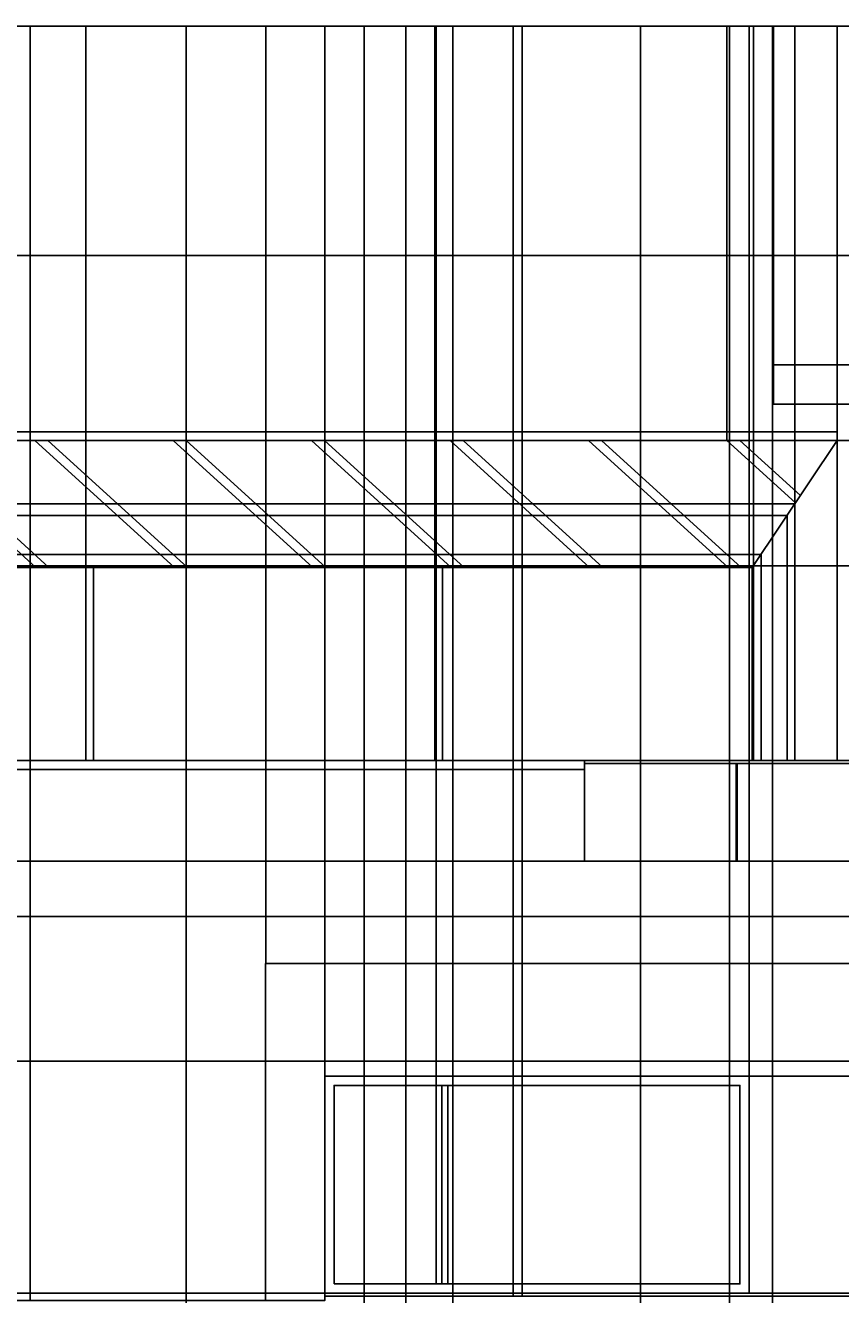
# Model space of a CAD drawing. Units: feet. Extents: x 2193 to 3502, y 890 to 1601.
# Tile 16 of 17: x 3069 to 3283, y 1268 to 1601. Entities that reach past the tile are written whole.
import ezdxf

# ---------------------------------------------------------------- set-up
doc = ezdxf.new("R2010")
doc.units = ezdxf.units.FT
doc.layers.add('A-ANNO-DIMS', color=2, linetype='Continuous', lineweight=18)
doc.layers.add('A-ELEV', color=7, linetype='Continuous', lineweight=25)
doc.styles.get("Standard").update_dxf_attribs({"font": 'arial.ttf'})
doc.dimstyles.get("Standard").update_dxf_attribs({"dimtxt": 0.18, "dimasz": 0.18, "dimexe": 0.18, "dimexo": 0.0625, "dimgap": 0.09, "dimtad": 0, "dimtih": 1, "dimtoh": 1, "dimdec": 0, "dimzin": 0, "dimdsep": 46, "dimlunit": 3, "dimtxsty": 'Standard', "dimcen": 0.09, "dimadec": 0, "dimazin": 0, "dimtfac": 1, "dimtdec": 0, "dimtofl": 0, "dimtmove": 0, "dimatfit": 3, "dimfxl": 1, "dimtolj": 1, "dimtzin": 0, "dimarcsym": 0})

# ---------------------------------------------------------------- blocks, each defined once
blk = doc.blocks.new('*D13')
at = {"layer": 'A-ANNO-DIMS', "color": 0, "lineweight": -2, "transparency": 16777216}
for p, q in [((2934.37, 950.89), (2934.37, 1601.47)), ((2934.55, 1601.29), (3186.64, 1601.29)), ((3439.51, 1601.29), (3187.43, 1601.29)), ((3439.69, 1541.11), (3439.69, 1601.47))]:
    blk.add_line(p, q, dxfattribs=at)
at = {"layer": 'A-ANNO-DIMS', "color": 0, "transparency": 16777216}
for points in [[(2934.55, 1601.32), (2934.55, 1601.26), (2934.37, 1601.29)], [(3439.51, 1601.32), (3439.51, 1601.26), (3439.69, 1601.29)]]:
    blk.add_solid(points, dxfattribs=at)
at = {"layer": 'Defpoints', "color": 0, "transparency": 16777216}
for p in [(3439.69, 1601.29), (3439.69, 1541.04), (2934.37, 950.82)]:
    blk.add_point(p, dxfattribs=at)
at = {"layer": 'A-ANNO-DIMS', "color": 0, "transparency": 16777216, "insert": (3187.03, 1601.29), "char_height": 0.18, "attachment_point": 5}
blk.add_mtext('\\A1;505.3', dxfattribs=at)
blk = doc.blocks.new('*D31')
at = {"layer": 'A-ANNO-DIMS', "color": 0, "lineweight": -2, "transparency": 16777216}
for p, q in [((2760.54, 1541.04), (3501.85, 1541.04)), ((3501.67, 1540.86), (3501.67, 1246.12)), ((3501.67, 951), (3501.67, 1245.75)), ((2762.27, 950.82), (3501.85, 950.82))]:
    blk.add_line(p, q, dxfattribs=at)
at = {"layer": 'A-ANNO-DIMS', "color": 0, "transparency": 16777216}
for points in [[(3501.64, 1540.86), (3501.7, 1540.86), (3501.67, 1541.04)], [(3501.64, 951), (3501.7, 951), (3501.67, 950.82)]]:
    blk.add_solid(points, dxfattribs=at)
at = {"layer": 'Defpoints', "color": 0, "transparency": 16777216}
for p in [(2760.47, 1541.04), (3501.67, 1541.04), (2762.2, 950.82)]:
    blk.add_point(p, dxfattribs=at)
at = {"layer": 'A-ANNO-DIMS', "color": 0, "transparency": 16777216, "insert": (3501.67, 1245.93), "char_height": 0.18, "attachment_point": 5}
blk.add_mtext('\\A1;590.2', dxfattribs=at)
blk = doc.blocks.new('*D43')
at = {"layer": 'A-ANNO-DIMS', "color": 0, "lineweight": -2, "transparency": 16777216}
for p, q in [((3265.39, 1512.46), (3265.39, 1601.47)), ((3265.57, 1601.29), (3273.35, 1601.29)), ((3281.9, 1601.29), (3274.12, 1601.29)), ((3282.08, 1502.14), (3282.08, 1601.47))]:
    blk.add_line(p, q, dxfattribs=at)
at = {"layer": 'A-ANNO-DIMS', "color": 0, "transparency": 16777216}
for points in [[(3265.57, 1601.32), (3265.57, 1601.26), (3265.39, 1601.29)], [(3281.9, 1601.32), (3281.9, 1601.26), (3282.08, 1601.29)]]:
    blk.add_solid(points, dxfattribs=at)
at = {"layer": 'Defpoints', "color": 0, "transparency": 16777216}
for p in [(3282.08, 1601.29), (3265.39, 1512.4), (3282.08, 1502.08)]:
    blk.add_point(p, dxfattribs=at)
at = {"layer": 'A-ANNO-DIMS', "color": 0, "transparency": 16777216, "insert": (3273.74, 1601.29), "char_height": 0.18, "attachment_point": 5}
blk.add_mtext('\\A1;16.69', dxfattribs=at)
blk = doc.blocks.new('*D44')
at = {"layer": 'A-ANNO-DIMS', "color": 0, "lineweight": -2, "transparency": 16777216}
for p, q in [((3282.08, 1502.14), (3282.08, 1601.47)), ((3282.26, 1601.29), (3330.07, 1601.29)), ((3378.67, 1601.29), (3330.86, 1601.29)), ((3378.85, 1502.14), (3378.85, 1601.47))]:
    blk.add_line(p, q, dxfattribs=at)
at = {"layer": 'A-ANNO-DIMS', "color": 0, "transparency": 16777216}
for points in [[(3282.26, 1601.32), (3282.26, 1601.26), (3282.08, 1601.29)], [(3378.67, 1601.32), (3378.67, 1601.26), (3378.85, 1601.29)]]:
    blk.add_solid(points, dxfattribs=at)
at = {"layer": 'Defpoints', "color": 0, "transparency": 16777216}
for p in [(3378.85, 1601.29), (3282.08, 1502.08), (3378.85, 1502.08)]:
    blk.add_point(p, dxfattribs=at)
at = {"layer": 'A-ANNO-DIMS', "color": 0, "transparency": 16777216, "insert": (3330.47, 1601.29), "char_height": 0.18, "attachment_point": 5}
blk.add_mtext('\\A1;96.77', dxfattribs=at)
blk = doc.blocks.new('*D48')
at = {"layer": 'A-ANNO-DIMS', "color": 0, "lineweight": -2, "transparency": 16777216}
for p, q in [((2965.72, 1494.87), (2965.72, 1601.47)), ((2965.9, 1601.29), (3123.44, 1601.29)), ((3281.9, 1601.29), (3124.36, 1601.29)), ((3282.08, 1494.87), (3282.08, 1601.47))]:
    blk.add_line(p, q, dxfattribs=at)
at = {"layer": 'A-ANNO-DIMS', "color": 0, "transparency": 16777216}
for points in [[(2965.9, 1601.32), (2965.9, 1601.26), (2965.72, 1601.29)], [(3281.9, 1601.32), (3281.9, 1601.26), (3282.08, 1601.29)]]:
    blk.add_solid(points, dxfattribs=at)
at = {"layer": 'Defpoints', "color": 0, "transparency": 16777216}
for p in [(3282.08, 1601.29), (2965.72, 1494.8), (3282.08, 1494.8)]:
    blk.add_point(p, dxfattribs=at)
at = {"layer": 'A-ANNO-DIMS', "color": 0, "transparency": 16777216, "insert": (3123.9, 1601.29), "char_height": 0.18, "attachment_point": 5}
blk.add_mtext('\\A1;316.36', dxfattribs=at)
blk = doc.blocks.new('*D50')
at = {"layer": 'A-ANNO-DIMS', "color": 0, "lineweight": -2, "transparency": 16777216}
for p, q in [((3260.1, 1459.67), (3260.1, 1601.47)), ((3260.28, 1601.29), (3270.7, 1601.29)), ((3281.9, 1601.29), (3271.49, 1601.29)), ((3282.08, 1492.58), (3282.08, 1601.47))]:
    blk.add_line(p, q, dxfattribs=at)
at = {"layer": 'A-ANNO-DIMS', "color": 0, "transparency": 16777216}
for points in [[(3260.28, 1601.32), (3260.28, 1601.26), (3260.1, 1601.29)], [(3281.9, 1601.32), (3281.9, 1601.26), (3282.08, 1601.29)]]:
    blk.add_solid(points, dxfattribs=at)
at = {"layer": 'Defpoints', "color": 0, "transparency": 16777216}
for p in [(3282.08, 1601.29), (3282.08, 1492.51), (3260.1, 1459.6)]:
    blk.add_point(p, dxfattribs=at)
at = {"layer": 'A-ANNO-DIMS', "color": 0, "transparency": 16777216, "insert": (3271.09, 1601.29), "char_height": 0.18, "attachment_point": 5}
blk.add_mtext('\\A1;21.98', dxfattribs=at)
blk = doc.blocks.new('*D51')
at = {"layer": 'A-ANNO-DIMS', "color": 0, "lineweight": -2, "transparency": 16777216}
for p, q in [((2965.78, 1492.51), (3501.85, 1492.51)), ((3501.67, 1492.33), (3501.67, 1476.24)), ((3501.67, 1459.78), (3501.67, 1475.88)), ((3001.96, 1459.6), (3501.85, 1459.6))]:
    blk.add_line(p, q, dxfattribs=at)
at = {"layer": 'A-ANNO-DIMS', "color": 0, "transparency": 16777216}
for points in [[(3501.64, 1492.33), (3501.7, 1492.33), (3501.67, 1492.51)], [(3501.64, 1459.78), (3501.7, 1459.78), (3501.67, 1459.6)]]:
    blk.add_solid(points, dxfattribs=at)
at = {"layer": 'Defpoints', "color": 0, "transparency": 16777216}
for p in [(2965.72, 1492.51), (3501.67, 1492.51), (3001.89, 1459.6)]:
    blk.add_point(p, dxfattribs=at)
at = {"layer": 'A-ANNO-DIMS', "color": 0, "transparency": 16777216, "insert": (3501.67, 1476.06), "char_height": 0.18, "attachment_point": 5}
blk.add_mtext('\\A1;32.91', dxfattribs=at)
blk = doc.blocks.new('*D54')
at = {"layer": 'A-ANNO-DIMS', "color": 0, "lineweight": -2, "transparency": 16777216}
for p, q in [((3002.38, 1408.54), (3002.38, 1601.47)), ((3002.56, 1601.29), (3043.2, 1601.29)), ((3084.62, 1601.29), (3043.99, 1601.29)), ((3084.8, 1408.54), (3084.8, 1601.47))]:
    blk.add_line(p, q, dxfattribs=at)
at = {"layer": 'A-ANNO-DIMS', "color": 0, "transparency": 16777216}
for points in [[(3002.56, 1601.32), (3002.56, 1601.26), (3002.38, 1601.29)], [(3084.62, 1601.32), (3084.62, 1601.26), (3084.8, 1601.29)]]:
    blk.add_solid(points, dxfattribs=at)
at = {"layer": 'Defpoints', "color": 0, "transparency": 16777216}
for p in [(3084.8, 1601.29), (3002.38, 1408.48), (3084.8, 1408.48)]:
    blk.add_point(p, dxfattribs=at)
at = {"layer": 'A-ANNO-DIMS', "color": 0, "transparency": 16777216, "insert": (3043.59, 1601.29), "char_height": 0.18, "attachment_point": 5}
blk.add_mtext('\\A1;82.42', dxfattribs=at)
blk = doc.blocks.new('*D55')
at = {"layer": 'A-ANNO-DIMS', "color": 0, "lineweight": -2, "transparency": 16777216}
for p, q in [((3084.8, 1408.54), (3084.8, 1601.47)), ((3084.98, 1601.29), (3130.23, 1601.29)), ((3176.26, 1601.29), (3131.01, 1601.29)), ((3176.44, 1408.54), (3176.44, 1601.47))]:
    blk.add_line(p, q, dxfattribs=at)
at = {"layer": 'A-ANNO-DIMS', "color": 0, "transparency": 16777216}
for points in [[(3084.98, 1601.32), (3084.98, 1601.26), (3084.8, 1601.29)], [(3176.26, 1601.32), (3176.26, 1601.26), (3176.44, 1601.29)]]:
    blk.add_solid(points, dxfattribs=at)
at = {"layer": 'Defpoints', "color": 0, "transparency": 16777216}
for p in [(3176.44, 1601.29), (3084.8, 1408.48), (3176.44, 1408.48)]:
    blk.add_point(p, dxfattribs=at)
at = {"layer": 'A-ANNO-DIMS', "color": 0, "transparency": 16777216, "insert": (3130.62, 1601.29), "char_height": 0.18, "attachment_point": 5}
blk.add_mtext('\\A1;91.63', dxfattribs=at)
blk = doc.blocks.new('*D56')
at = {"layer": 'A-ANNO-DIMS', "color": 0, "lineweight": -2, "transparency": 16777216}
for p, q in [((3176.44, 1408.54), (3176.44, 1601.47)), ((3176.62, 1601.29), (3217.87, 1601.29)), ((3259.92, 1601.29), (3218.66, 1601.29)), ((3260.1, 1408.54), (3260.1, 1601.47))]:
    blk.add_line(p, q, dxfattribs=at)
at = {"layer": 'A-ANNO-DIMS', "color": 0, "transparency": 16777216}
for points in [[(3176.62, 1601.32), (3176.62, 1601.26), (3176.44, 1601.29)], [(3259.92, 1601.32), (3259.92, 1601.26), (3260.1, 1601.29)]]:
    blk.add_solid(points, dxfattribs=at)
at = {"layer": 'Defpoints', "color": 0, "transparency": 16777216}
for p in [(3260.1, 1601.29), (3176.44, 1408.48), (3260.1, 1408.48)]:
    blk.add_point(p, dxfattribs=at)
at = {"layer": 'A-ANNO-DIMS', "color": 0, "transparency": 16777216, "insert": (3218.27, 1601.29), "char_height": 0.18, "attachment_point": 5}
blk.add_mtext('\\A1;83.66', dxfattribs=at)
blk = doc.blocks.new('*D57')
at = {"layer": 'A-ANNO-DIMS', "color": 0, "lineweight": -2, "transparency": 16777216}
for p, q in [((3260.1, 1408.54), (3260.1, 1601.47)), ((3260.28, 1601.29), (3265.07, 1601.29)), ((3270.78, 1601.29), (3265.98, 1601.29)), ((3270.96, 1408.54), (3270.96, 1601.47))]:
    blk.add_line(p, q, dxfattribs=at)
at = {"layer": 'A-ANNO-DIMS', "color": 0, "transparency": 16777216}
for points in [[(3260.28, 1601.32), (3260.28, 1601.26), (3260.1, 1601.29)], [(3270.78, 1601.32), (3270.78, 1601.26), (3270.96, 1601.29)]]:
    blk.add_solid(points, dxfattribs=at)
at = {"layer": 'Defpoints', "color": 0, "transparency": 16777216}
for p in [(3270.96, 1601.29), (3260.1, 1408.48), (3270.96, 1408.48)]:
    blk.add_point(p, dxfattribs=at)
at = {"layer": 'A-ANNO-DIMS', "color": 0, "transparency": 16777216, "insert": (3265.53, 1601.29), "char_height": 0.18, "attachment_point": 5}
blk.add_mtext('\\A1;10.855', dxfattribs=at)
blk = doc.blocks.new('*D59')
at = {"layer": 'A-ANNO-DIMS', "color": 0, "lineweight": -2, "transparency": 16777216}
for p, q in [((2974.12, 1329.64), (2974.12, 1601.47)), ((2974.3, 1601.29), (3021.89, 1601.29)), ((3069.93, 1601.29), (3022.33, 1601.29)), ((3070.11, 1329.64), (3070.11, 1601.47))]:
    blk.add_line(p, q, dxfattribs=at)
at = {"layer": 'A-ANNO-DIMS', "color": 0, "transparency": 16777216}
for points in [[(2974.3, 1601.32), (2974.3, 1601.26), (2974.12, 1601.29)], [(3069.93, 1601.32), (3069.93, 1601.26), (3070.11, 1601.29)]]:
    blk.add_solid(points, dxfattribs=at)
at = {"layer": 'Defpoints', "color": 0, "transparency": 16777216}
for p in [(3070.11, 1601.29), (2974.12, 1329.58), (3070.11, 1329.58)]:
    blk.add_point(p, dxfattribs=at)
at = {"layer": 'A-ANNO-DIMS', "color": 0, "transparency": 16777216, "insert": (3022.11, 1601.29), "char_height": 0.18, "attachment_point": 5}
blk.add_mtext('\\A1;96', dxfattribs=at)
blk = doc.blocks.new('*D60')
at = {"layer": 'A-ANNO-DIMS', "color": 0, "lineweight": -2, "transparency": 16777216}
for p, q in [((3070.17, 1329.58), (3501.85, 1329.58)), ((3501.67, 1329.4), (3501.67, 1299.3)), ((3501.67, 1268.84), (3501.67, 1298.94)), ((3070.17, 1268.66), (3501.85, 1268.66))]:
    blk.add_line(p, q, dxfattribs=at)
at = {"layer": 'A-ANNO-DIMS', "color": 0, "transparency": 16777216}
for points in [[(3501.64, 1329.4), (3501.7, 1329.4), (3501.67, 1329.58)], [(3501.64, 1268.84), (3501.7, 1268.84), (3501.67, 1268.66)]]:
    blk.add_solid(points, dxfattribs=at)
at = {"layer": 'Defpoints', "color": 0, "transparency": 16777216}
for p in [(3070.11, 1329.58), (3501.67, 1329.58), (3070.11, 1268.66)]:
    blk.add_point(p, dxfattribs=at)
at = {"layer": 'A-ANNO-DIMS', "color": 0, "transparency": 16777216, "insert": (3501.67, 1299.12), "char_height": 0.18, "attachment_point": 5}
blk.add_mtext('\\A1;60.92', dxfattribs=at)
blk = doc.blocks.new('*D71')
at = {"layer": 'A-ANNO-DIMS', "color": 0, "lineweight": -2, "transparency": 16777216}
for p, q in [((3132, 1355.28), (3132, 1601.47)), ((3132.18, 1601.29), (3216.71, 1601.29)), ((3302.02, 1601.29), (3217.48, 1601.29)), ((3302.2, 1355.28), (3302.2, 1601.47))]:
    blk.add_line(p, q, dxfattribs=at)
at = {"layer": 'A-ANNO-DIMS', "color": 0, "transparency": 16777216}
for points in [[(3132.18, 1601.32), (3132.18, 1601.26), (3132, 1601.29)], [(3302.02, 1601.32), (3302.02, 1601.26), (3302.2, 1601.29)]]:
    blk.add_solid(points, dxfattribs=at)
at = {"layer": 'Defpoints', "color": 0, "transparency": 16777216}
for p in [(3302.2, 1601.29), (3132, 1355.22), (3302.2, 1355.22)]:
    blk.add_point(p, dxfattribs=at)
at = {"layer": 'A-ANNO-DIMS', "color": 0, "transparency": 16777216, "insert": (3217.1, 1601.29), "char_height": 0.18, "attachment_point": 5}
blk.add_mtext('\\A1;170.2', dxfattribs=at)
blk = doc.blocks.new('*D73')
at = {"layer": 'A-ANNO-DIMS', "color": 0, "lineweight": -2, "transparency": 16777216}
for p, q in [((3147.5, 1325.73), (3147.5, 1601.47)), ((3147.68, 1601.29), (3202.79, 1601.29)), ((3258.8, 1601.29), (3203.7, 1601.29)), ((3258.98, 1325.73), (3258.98, 1601.47))]:
    blk.add_line(p, q, dxfattribs=at)
at = {"layer": 'A-ANNO-DIMS', "color": 0, "transparency": 16777216}
for points in [[(3147.68, 1601.32), (3147.68, 1601.26), (3147.5, 1601.29)], [(3258.8, 1601.32), (3258.8, 1601.26), (3258.98, 1601.29)]]:
    blk.add_solid(points, dxfattribs=at)
at = {"layer": 'Defpoints', "color": 0, "transparency": 16777216}
for p in [(3258.98, 1601.29), (3147.5, 1325.67), (3258.98, 1325.67)]:
    blk.add_point(p, dxfattribs=at)
at = {"layer": 'A-ANNO-DIMS', "color": 0, "transparency": 16777216, "insert": (3203.24, 1601.29), "char_height": 0.18, "attachment_point": 5}
blk.add_mtext('\\A1;111.48', dxfattribs=at)
blk = doc.blocks.new('*D74')
at = {"layer": 'A-ANNO-DIMS', "color": 0, "lineweight": -2, "transparency": 16777216}
for p, q in [((3147.5, 1325.73), (3147.5, 1601.47)), ((3147.68, 1601.29), (3161.68, 1601.29)), ((3176.61, 1601.29), (3162.61, 1601.29)), ((3176.79, 1323.29), (3176.79, 1601.47))]:
    blk.add_line(p, q, dxfattribs=at)
at = {"layer": 'A-ANNO-DIMS', "color": 0, "transparency": 16777216}
for points in [[(3147.68, 1601.32), (3147.68, 1601.26), (3147.5, 1601.29)], [(3176.61, 1601.32), (3176.61, 1601.26), (3176.79, 1601.29)]]:
    blk.add_solid(points, dxfattribs=at)
at = {"layer": 'Defpoints', "color": 0, "transparency": 16777216}
for p in [(3176.79, 1601.29), (3147.5, 1325.67), (3176.79, 1323.22)]:
    blk.add_point(p, dxfattribs=at)
at = {"layer": 'A-ANNO-DIMS', "color": 0, "transparency": 16777216, "insert": (3162.15, 1601.29), "char_height": 0.18, "attachment_point": 5}
blk.add_mtext('\\A1;29.286', dxfattribs=at)
blk = doc.blocks.new('*D75')
at = {"layer": 'A-ANNO-DIMS', "color": 0, "lineweight": -2, "transparency": 16777216}
for p, q in [((3259.05, 1325.67), (3501.85, 1325.67)), ((3501.67, 1325.49), (3501.67, 1297.35)), ((3501.67, 1268.84), (3501.67, 1296.98)), ((3259.05, 1268.66), (3501.85, 1268.66))]:
    blk.add_line(p, q, dxfattribs=at)
at = {"layer": 'A-ANNO-DIMS', "color": 0, "transparency": 16777216}
for points in [[(3501.64, 1325.49), (3501.7, 1325.49), (3501.67, 1325.67)], [(3501.64, 1268.84), (3501.7, 1268.84), (3501.67, 1268.66)]]:
    blk.add_solid(points, dxfattribs=at)
at = {"layer": 'Defpoints', "color": 0, "transparency": 16777216}
for p in [(3258.98, 1325.67), (3501.67, 1325.67), (3258.98, 1268.66)]:
    blk.add_point(p, dxfattribs=at)
at = {"layer": 'A-ANNO-DIMS', "color": 0, "transparency": 16777216, "insert": (3501.67, 1297.16), "char_height": 0.18, "attachment_point": 5}
blk.add_mtext('\\A1;57.01', dxfattribs=at)
blk = doc.blocks.new('*D84')
at = {"layer": 'A-ANNO-DIMS', "color": 0, "lineweight": -2, "transparency": 16777216}
for p, q in [((3196.98, 1267.98), (3196.98, 1601.47)), ((3197.16, 1601.29), (3197.76, 1601.29)), ((3199.15, 1601.29), (3198.55, 1601.29)), ((3199.33, 1267.98), (3199.33, 1601.47))]:
    blk.add_line(p, q, dxfattribs=at)
at = {"layer": 'A-ANNO-DIMS', "color": 0, "transparency": 16777216}
for points in [[(3197.16, 1601.32), (3197.16, 1601.26), (3196.98, 1601.29)], [(3199.15, 1601.32), (3199.15, 1601.26), (3199.33, 1601.29)]]:
    blk.add_solid(points, dxfattribs=at)
at = {"layer": 'Defpoints', "color": 0, "transparency": 16777216}
for p in [(3199.33, 1601.29), (3196.98, 1267.92), (3199.33, 1267.92)]:
    blk.add_point(p, dxfattribs=at)
at = {"layer": 'A-ANNO-DIMS', "color": 0, "transparency": 16777216, "insert": (3198.15, 1601.29), "char_height": 0.18, "attachment_point": 5}
blk.add_mtext('\\A1;2.358', dxfattribs=at)
blk = doc.blocks.new('*D97')
at = {"layer": 'A-ANNO-DIMS', "color": 0, "lineweight": -2, "transparency": 16777216}
for p, q in [((3111.13, 1032.26), (3111.13, 1601.47)), ((3111.31, 1601.29), (3207.6, 1601.29)), ((3304.79, 1601.29), (3208.51, 1601.29)), ((3304.97, 1032.26), (3304.97, 1601.47))]:
    blk.add_line(p, q, dxfattribs=at)
at = {"layer": 'A-ANNO-DIMS', "color": 0, "transparency": 16777216}
for points in [[(3111.31, 1601.32), (3111.31, 1601.26), (3111.13, 1601.29)], [(3304.79, 1601.32), (3304.79, 1601.26), (3304.97, 1601.29)]]:
    blk.add_solid(points, dxfattribs=at)
at = {"layer": 'Defpoints', "color": 0, "transparency": 16777216}
for p in [(3304.97, 1601.29), (3111.13, 1032.19), (3304.97, 1032.19)]:
    blk.add_point(p, dxfattribs=at)
at = {"layer": 'A-ANNO-DIMS', "color": 0, "transparency": 16777216, "insert": (3208.05, 1601.29), "char_height": 0.18, "attachment_point": 5}
blk.add_mtext('\\A1;193.84', dxfattribs=at)
blk = doc.blocks.new('*D100')
at = {"layer": 'A-ANNO-DIMS', "color": 0, "lineweight": -2, "transparency": 16777216}
for p, q in [((3168.83, 1055.37), (3168.83, 1601.47)), ((3169.01, 1601.29), (3216.57, 1601.29)), ((3264.92, 1601.29), (3217.36, 1601.29)), ((3265.1, 1055.37), (3265.1, 1601.47))]:
    blk.add_line(p, q, dxfattribs=at)
at = {"layer": 'A-ANNO-DIMS', "color": 0, "transparency": 16777216}
for points in [[(3169.01, 1601.32), (3169.01, 1601.26), (3168.83, 1601.29)], [(3264.92, 1601.32), (3264.92, 1601.26), (3265.1, 1601.29)]]:
    blk.add_solid(points, dxfattribs=at)
at = {"layer": 'Defpoints', "color": 0, "transparency": 16777216}
for p in [(3265.1, 1601.29), (3168.83, 1055.31), (3265.1, 1055.31)]:
    blk.add_point(p, dxfattribs=at)
at = {"layer": 'A-ANNO-DIMS', "color": 0, "transparency": 16777216, "insert": (3216.97, 1601.29), "char_height": 0.18, "attachment_point": 5}
blk.add_mtext('\\A1;96.27', dxfattribs=at)
blk = doc.blocks.new('*D104')
at = {"layer": 'A-ANNO-DIMS', "color": 0, "lineweight": -2, "transparency": 16777216}
for p, q in [((3157.83, 1001.2), (3157.83, 1601.47)), ((3158.01, 1601.29), (3169.1, 1601.29)), ((3180.99, 1601.29), (3169.89, 1601.29)), ((3181.17, 1001.2), (3181.17, 1601.47))]:
    blk.add_line(p, q, dxfattribs=at)
at = {"layer": 'A-ANNO-DIMS', "color": 0, "transparency": 16777216}
for points in [[(3158.01, 1601.32), (3158.01, 1601.26), (3157.83, 1601.29)], [(3180.99, 1601.32), (3180.99, 1601.26), (3181.17, 1601.29)]]:
    blk.add_solid(points, dxfattribs=at)
at = {"layer": 'Defpoints', "color": 0, "transparency": 16777216}
for p in [(3181.17, 1601.29), (3157.83, 1001.13), (3181.17, 1001.13)]:
    blk.add_point(p, dxfattribs=at)
at = {"layer": 'A-ANNO-DIMS', "color": 0, "transparency": 16777216, "insert": (3169.5, 1601.29), "char_height": 0.18, "attachment_point": 5}
blk.add_mtext('\\A1;23.34', dxfattribs=at)
blk = doc.blocks.new('*D106')
at = {"layer": 'A-ANNO-DIMS', "color": 0, "lineweight": -2, "transparency": 16777216}
for p, q in [((3230.44, 1001.2), (3230.44, 1601.47)), ((3230.62, 1601.29), (3241.72, 1601.29)), ((3253.6, 1601.29), (3242.51, 1601.29)), ((3253.78, 1001.2), (3253.78, 1601.47))]:
    blk.add_line(p, q, dxfattribs=at)
at = {"layer": 'A-ANNO-DIMS', "color": 0, "transparency": 16777216}
for points in [[(3230.62, 1601.32), (3230.62, 1601.26), (3230.44, 1601.29)], [(3253.6, 1601.32), (3253.6, 1601.26), (3253.78, 1601.29)]]:
    blk.add_solid(points, dxfattribs=at)
at = {"layer": 'Defpoints', "color": 0, "transparency": 16777216}
for p in [(3253.78, 1601.29), (3230.44, 1001.13), (3253.78, 1001.13)]:
    blk.add_point(p, dxfattribs=at)
at = {"layer": 'A-ANNO-DIMS', "color": 0, "transparency": 16777216, "insert": (3242.11, 1601.29), "char_height": 0.18, "attachment_point": 5}
blk.add_mtext('\\A1;23.34', dxfattribs=at)
blk = doc.blocks.new('*D129')
at = {"layer": 'A-ANNO-DIMS', "color": 0, "lineweight": -2, "transparency": 16777216}
for p, q in [((3253.14, 1492.58), (3253.14, 1601.47)), ((3253.32, 1601.29), (3267.22, 1601.29)), ((3281.9, 1601.29), (3268.01, 1601.29)), ((3282.08, 1492.58), (3282.08, 1601.47))]:
    blk.add_line(p, q, dxfattribs=at)
at = {"layer": 'A-ANNO-DIMS', "color": 0, "transparency": 16777216}
for points in [[(3253.32, 1601.32), (3253.32, 1601.26), (3253.14, 1601.29)], [(3281.9, 1601.32), (3281.9, 1601.26), (3282.08, 1601.29)]]:
    blk.add_solid(points, dxfattribs=at)
at = {"layer": 'Defpoints', "color": 0, "transparency": 16777216}
for p in [(3282.08, 1601.29), (3253.14, 1492.51), (3282.08, 1492.51)]:
    blk.add_point(p, dxfattribs=at)
at = {"layer": 'A-ANNO-DIMS', "color": 0, "transparency": 16777216, "insert": (3267.61, 1601.29), "char_height": 0.18, "attachment_point": 5}
blk.add_mtext('\\A1;28.94', dxfattribs=at)

msp = doc.modelspace()

# ---------------------------------------------------------------- linework, layer by layer
at = {"layer": 'A-ELEV'}
for p, q in [((3439.6901, 1502.0763), (3265.3903, 1502.0763)), ((3035.0107, 1492.5146), (3071.6737, 1459.1592)), ((3038.4293, 1492.5146), (3075.0923, 1459.1592)), ((3071.3656, 1492.5146), (3108.0286, 1459.1592)), ((3074.7841, 1492.5146), (3111.4472, 1459.1592)), ((3107.7204, 1492.5146), (3144.3834, 1459.1592)), ((3111.139, 1492.5146), (3147.802, 1459.1592)), ((3144.0752, 1492.5146), (3180.7382, 1459.1592)), ((3147.4938, 1492.5146), (3184.1568, 1459.1592)), ((3180.43, 1492.5146), (3217.093, 1459.1592)), ((3183.8486, 1492.5146), (3220.5116, 1459.1592)), ((3216.7849, 1492.5146), (3253.4479, 1459.1592)), ((3220.2034, 1492.5146), (3256.8664, 1459.1592)), ((3253.1397, 1492.5146), (3271.1424, 1476.1361)), ((3256.5583, 1492.5146), (3272.4345, 1478.0707)), ((3259.8035, 1459.1592), (3282.0816, 1492.5146)), ((3270.9554, 1475.8561), (2984.0301, 1475.8561)), ((3268.9492, 1472.8525), (2987.3316, 1472.8525)), ((3262.1063, 1462.6071), (2998.5929, 1462.6071)), ((3260.1002, 1459.6035), (3001.8944, 1459.6035)), ((3002.3827, 1459.1592), (3259.8035, 1459.1592)), ((3259.8035, 1408.4814), (3259.8035, 1459.1592)), ((3215.7583, 1367.5739), (3325.5011, 1367.5739)), ((3131.9988, 1355.2199), (3302.1981, 1355.2199))]:
    msp.add_line(p, q, dxfattribs=at)
for points in [[(3282.0816, 1502.0763), (3265.3903, 1502.0763), (3265.3903, 1512.3957), (3439.6901, 1512.3957), (3439.6901, 1502.0763)], [(3270.9554, 1475.8561), (3270.9554, 1408.4814), (3268.9492, 1408.4814), (3268.9492, 1472.8525)], [(3262.1063, 1462.6071), (3262.1063, 1408.4814), (3260.1002, 1408.4814), (3260.1002, 1459.6035)], [(3215.7583, 1408.4814), (2934.3742, 1408.4814)], [(2935.5399, 1406.15), (3215.7583, 1406.15), (3215.7583, 1407.3157)], [(3215.7583, 1408.4814), (3215.7583, 1407.3157)], [(3215.7583, 1408.4814), (3378.7894, 1408.4814)], [(3378.7894, 1407.7384), (3215.7583, 1407.7384)], [(3215.7583, 1382.0763), (3215.7583, 1407.3157)], [(3255.8092, 1407.7384), (3255.8092, 1382.0763), (3255.5595, 1382.0763), (3255.5595, 1407.7384)], [(3425.1877, 1367.5739), (2954.2649, 1367.5739), (2954.2649, 1382.0763), (3439.6901, 1382.0763), (3439.6901, 1367.5739)], [(2974.116, 1367.5739), (3215.7583, 1367.5739)], [(3070.1101, 1367.5739), (3070.1101, 1266.7092), (3131.9988, 1266.7092), (3131.9988, 1355.2199)], [(3378.849, 1267.9169), (3147.5022, 1267.9169), (3147.5022, 1268.6599), (3378.849, 1268.6599)]]:
    msp.add_lwpolyline(points, dxfattribs=at)
for points in [[(3378.7894, 1408.4814), (3282.0816, 1408.4814), (3282.0816, 1502.0763), (3378.7894, 1502.0763)], [(3282.0816, 1494.8043), (2965.7197, 1494.8043), (2965.7197, 1492.5146), (3282.0816, 1492.5146)], [(3084.8031, 1459.1592), (3086.8092, 1459.1592), (3086.8092, 1408.4814), (3084.8031, 1408.4814)], [(3176.4359, 1459.1592), (3178.442, 1459.1592), (3178.442, 1408.4814), (3176.4359, 1408.4814)], [(2974.116, 1268.6599), (3070.1101, 1268.6599), (3070.1101, 1329.5765), (2974.116, 1329.5765)], [(3147.5022, 1268.6599), (3258.9838, 1268.6599), (3258.9838, 1325.6699), (3147.5022, 1325.6699)], [(3149.9473, 1271.105), (3256.5386, 1271.105), (3256.5386, 1323.2248), (3149.9473, 1323.2248)], [(3176.7885, 1323.2248), (3178.3021, 1323.2248), (3178.3021, 1271.105), (3176.7885, 1271.105)], [(3178.3021, 1323.2248), (3179.8157, 1323.2248), (3179.8157, 1271.105), (3178.3021, 1271.105)], [(2974.116, 1266.7092), (3147.5022, 1266.7092), (3147.5022, 1268.6599), (2974.116, 1268.6599)]]:
    msp.add_lwpolyline(points, close=True, dxfattribs=at)

# ---------------------------------------------------------------- dimensions: what is measured, and where the dimension line sits
at = {"layer": 'A-ANNO-DIMS'}
for base, p1, p2, override, picture, middle in [((3439.6901, 1601.2941), (2934.3742, 950.8228), (3439.6901, 1541.0441), {"dimdec": 1, "dimlfac": 1, "dimrnd": 0, "dimzin": 0, "dimdsep": 46, "dimlunit": 2}, '*D13', (3187.0321, 1601.2941)), ((3282.0816, 1601.2941), (2965.7197, 1494.8043), (3282.0816, 1494.8043), {"dimdec": 2, "dimlfac": 1, "dimrnd": 0, "dimzin": 0, "dimdsep": 46, "dimlunit": 2}, '*D48', (3123.9006, 1601.2941)), ((3070.1101, 1601.2941), (2974.116, 1329.5765), (3070.1101, 1329.5765), {"dimdec": 0, "dimlfac": 1, "dimrnd": 0, "dimzin": 0, "dimdsep": 46, "dimlunit": 2}, '*D59', (3022.113, 1601.2941)), ((3084.8031, 1601.2941), (3002.3827, 1408.4814), (3084.8031, 1408.4814), {"dimdec": 2, "dimlfac": 1, "dimrnd": 0, "dimzin": 0, "dimdsep": 46, "dimlunit": 2}, '*D54', (3043.5929, 1601.2941)), ((3176.4359, 1601.2941), (3084.8031, 1408.4814), (3176.4359, 1408.4814), {"dimdec": 2, "dimlfac": 1, "dimrnd": 0, "dimzin": 0, "dimdsep": 46, "dimlunit": 2}, '*D55', (3130.6195, 1601.2941)), ((3304.9731, 1601.2941), (3111.1302, 1032.1935), (3304.9731, 1032.1935), {"dimdec": 2, "dimlfac": 1, "dimrnd": 0, "dimzin": 0, "dimdsep": 46, "dimlunit": 2}, '*D97', (3208.0516, 1601.2941)), ((3302.1981, 1601.2941), (3131.9988, 1355.2199), (3302.1981, 1355.2199), {"dimdec": 1, "dimlfac": 1, "dimrnd": 0, "dimzin": 0, "dimdsep": 46, "dimlunit": 2}, '*D71', (3217.0985, 1601.2941)), ((3258.9838, 1601.2941), (3147.5022, 1325.6699), (3258.9838, 1325.6699), {"dimdec": 2, "dimlfac": 1, "dimrnd": 0, "dimzin": 0, "dimdsep": 46, "dimlunit": 2}, '*D73', (3203.243, 1601.2941)), ((3176.7885, 1601.2941), (3147.5022, 1325.6699), (3176.7885, 1323.2248), {"dimdec": 3, "dimlfac": 1, "dimrnd": 0, "dimzin": 0, "dimdsep": 46, "dimlunit": 2}, '*D74', (3162.1453, 1601.2941)), ((3181.1661, 1601.2941), (3157.8263, 1001.1334), (3181.1661, 1001.1334), {"dimdec": 2, "dimlfac": 1, "dimrnd": 0, "dimzin": 0, "dimdsep": 46, "dimlunit": 2}, '*D104', (3169.4962, 1601.2941)), ((3265.1012, 1601.2941), (3168.8336, 1055.3069), (3265.1012, 1055.3069), {"dimdec": 2, "dimlfac": 1, "dimrnd": 0, "dimzin": 0, "dimdsep": 46, "dimlunit": 2}, '*D100', (3216.9674, 1601.2941)), ((3260.1002, 1601.2941), (3176.4359, 1408.4814), (3260.1002, 1408.4814), {"dimdec": 2, "dimlfac": 1, "dimrnd": 0, "dimzin": 0, "dimdsep": 46, "dimlunit": 2}, '*D56', (3218.268, 1601.2941)), ((3199.3336, 1601.2941), (3196.9758, 1267.9169), (3199.3336, 1267.9169), {"dimdec": 3, "dimlfac": 1, "dimrnd": 0, "dimzin": 0, "dimdsep": 46, "dimlunit": 2}, '*D84', (3198.1547, 1601.2941)), ((3253.781, 1601.2941), (3230.4412, 1001.1334), (3253.781, 1001.1334), {"dimdec": 2, "dimlfac": 1, "dimrnd": 0, "dimzin": 0, "dimdsep": 46, "dimlunit": 2}, '*D106', (3242.1111, 1601.2941)), ((3282.0816, 1601.2941), (3253.1397, 1492.5146), (3282.0816, 1492.5146), {"dimdec": 2, "dimlfac": 1, "dimrnd": 0, "dimzin": 0, "dimdsep": 46, "dimlunit": 2}, '*D129', (3267.6106, 1601.2941)), ((3282.0816, 1601.2941), (3260.1002, 1459.6035), (3282.0816, 1492.5146), {"dimdec": 2, "dimlfac": 1, "dimrnd": 0, "dimzin": 0, "dimdsep": 46, "dimlunit": 2}, '*D50', (3271.0909, 1601.2941)), ((3270.9554, 1601.2941), (3260.1002, 1408.4814), (3270.9554, 1408.4814), {"dimdec": 3, "dimlfac": 1, "dimrnd": 0, "dimzin": 0, "dimdsep": 46, "dimlunit": 2}, '*D57', (3265.5278, 1601.2941)), ((3282.0816, 1601.2941), (3265.3903, 1512.3957), (3282.0816, 1502.0763), {"dimdec": 2, "dimlfac": 1, "dimrnd": 0, "dimzin": 0, "dimdsep": 46, "dimlunit": 2}, '*D43', (3273.736, 1601.2941)), ((3378.849, 1601.2941), (3282.0816, 1502.0763), (3378.849, 1502.0763), {"dimdec": 2, "dimlfac": 1, "dimrnd": 0, "dimzin": 0, "dimdsep": 46, "dimlunit": 2}, '*D44', (3330.4653, 1601.2941))]:
    dim = msp.add_linear_dim(base=base, p1=p1, p2=p2, dimstyle='Standard', override=override, dxfattribs=at)
    dim.commit()
    dim.dimension.update_dxf_attribs({"geometry": picture, "text_midpoint": middle})
for base, p1, p2, override, picture, middle in [((3501.6716, 1541.0441), (2762.2048, 950.8228), (2760.4733, 1541.0441), {"dimdec": 1, "dimlfac": 1, "dimrnd": 0, "dimzin": 0, "dimdsep": 46, "dimlunit": 2}, '*D31', (3501.6716, 1245.9334)), ((3501.6716, 1492.5146), (3001.8944, 1459.6035), (2965.7197, 1492.5146), {"dimdec": 2, "dimlfac": 1, "dimrnd": 0, "dimzin": 0, "dimdsep": 46, "dimlunit": 2}, '*D51', (3501.6716, 1476.0591)), ((3501.6716, 1329.5765), (3070.1101, 1268.6599), (3070.1101, 1329.5765), {"dimdec": 2, "dimlfac": 1, "dimrnd": 0, "dimzin": 0, "dimdsep": 46, "dimlunit": 2}, '*D60', (3501.6716, 1299.1182)), ((3501.6716, 1325.6699), (3258.9838, 1268.6599), (3258.9838, 1325.6699), {"dimdec": 2, "dimlfac": 1, "dimrnd": 0, "dimzin": 0, "dimdsep": 46, "dimlunit": 2}, '*D75', (3501.6716, 1297.1649))]:
    dim = msp.add_linear_dim(base=base, p1=p1, p2=p2, angle=90, dimstyle='Standard', override=override, dxfattribs=at)
    dim.commit()
    dim.dimension.update_dxf_attribs({"geometry": picture, "text_midpoint": middle})

doc.saveas('drawing.dxf')
